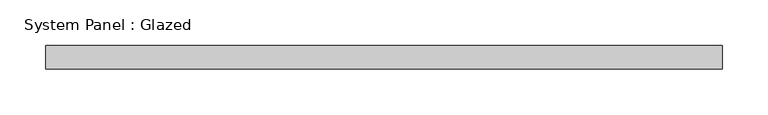
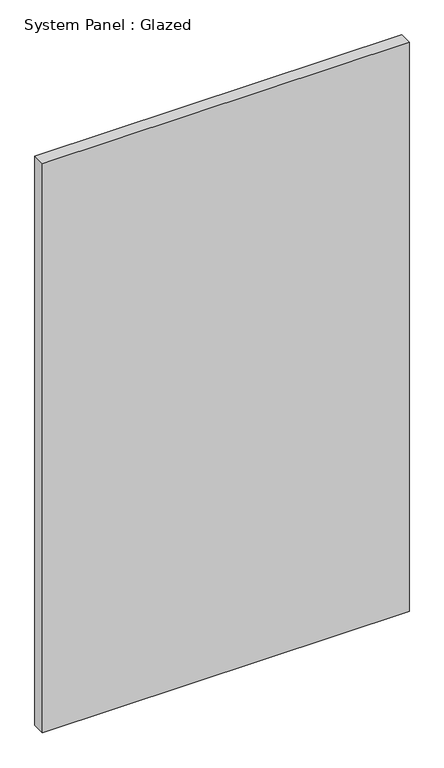
"""IFC4 building model written with IfcOpenShell, lengths in millimetres: plate geometry, System Panel : Glazed."""

from ifc_helpers import new_model, si_unit, origin, origin_with_axes, place, context, project, spatial, polyline, outline, extrude, source, transform, mapped, element, save


def system_panel_glazed_e62deb46(model_context):
    return source(origin(), model_context, "Body", "SweptSolid", [
        extrude(outline(polyline([(369.22075, 19.05), (-369.22075, 19.05), (-369.22075, 44.45), (369.22075, 44.45), (369.22075, 19.05)])), origin_with_axes(), (0.0, 0.0, 1.0), 1211.961),
    ])


if __name__ == "__main__":
    model = new_model("IFC4")
    model_context = context("Model", 3, world=origin())
    ifc_project = project(units=[si_unit("LENGTHUNIT", "METRE", prefix="MILLI")], contexts=[model_context])
    site = spatial("IfcSite", under=ifc_project)
    building = spatial("IfcBuilding", under=site)
    placement = place(None, origin())
    system_panel_glazed_shape = system_panel_glazed_e62deb46(model_context)
    element("IfcPlate", 1, ObjectType="System Panel : Glazed", at=placement, inside=building, context=model_context, shape_type="MappedRepresentation", body=[
        mapped(system_panel_glazed_shape, transform((0.0, 0.0, 0.0), x_axis=(1.0, 0.0, 0.0), y_axis=(0.0, 1.0, 0.0), z_axis=(0.0, 0.0, 1.0))),
    ])
    save(model, "model.ifc")

# Revit data of these elements
# Type "System Panel : Glazed"
#   Construction Type Id = "GSP4R"
#   Analytic Construction = "1/8 in Pilkington single glazing"
#   Visual Light Transmittance = 0.9
#   Solar Heat Gain Coefficient = 0.86
#   Heat Transfer Coefficient (U) = 1.18115 BTU/(h·ft²·°F)
#   Define Thermal Properties by = 1
# Element 1 (IfcPlate, "System Panel : Glazed")
#   Materials on its faces: "Glass"
# Materials
#   "Glass": class "Glass", colour RGB 0 128 192, transparency 0.75, Description = "Soda Lime Glass", Cost = 0
